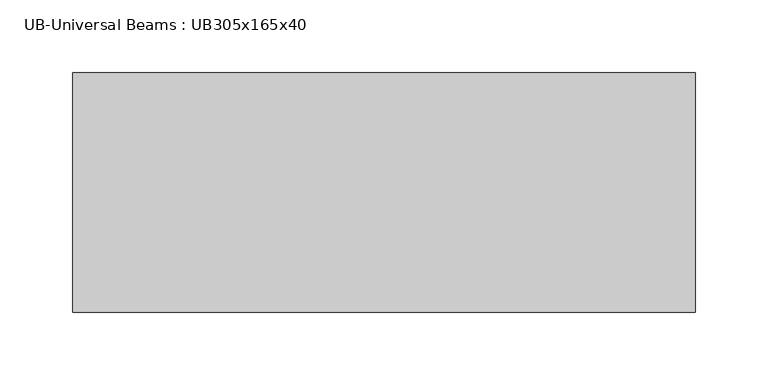
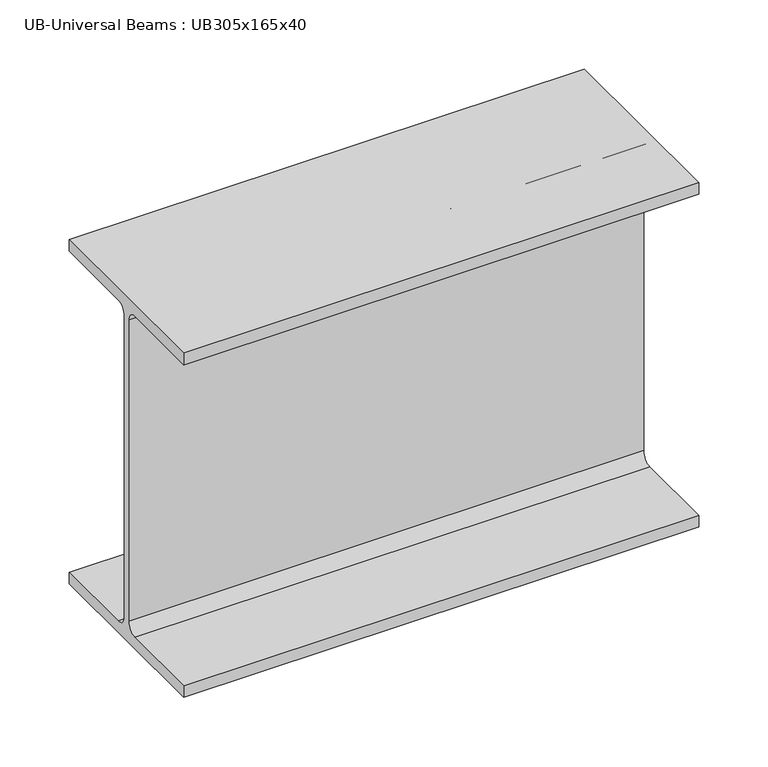
"""IFC4 building model written with IfcOpenShell, lengths in millimetres: beam geometry, UB-Universal Beams : UB305x165x40."""

from ifc_helpers import new_model, si_unit, point, frame, frame_2d, origin, place, context, project, spatial, polyline, circle_curve, trimmed, segment, composite_curve, outline, extrude, source, transform, mapped, element, save


def ub_universal_beams_ub305x165x40_c2ddfea9(model_context):
    return source(origin(), model_context, "Body", "SweptSolid", [
        extrude(outline(composite_curve([segment(polyline([(-82.5, -141.5), (-11.9, -141.5)]), True, "CONTINUOUS"), segment(trimmed(circle_curve(frame_2d((-11.9, -132.6)), 8.9), [point((-11.9, -141.5))], [point((-3.0, -132.6))], True, "CARTESIAN"), True, "CONTINUOUS"), segment(polyline([(-3.0, -132.6), (-3.0, 132.6)]), True, "CONTINUOUS"), segment(trimmed(circle_curve(frame_2d((-11.9, 132.6)), 8.9), [point((-3.0, 132.6))], [point((-11.9, 141.5))], True, "CARTESIAN"), True, "CONTINUOUS"), segment(polyline([(-11.9, 141.5), (-82.5, 141.5), (-82.5, 151.7), (82.5, 151.7), (82.5, 141.5), (11.9, 141.5)]), True, "CONTINUOUS"), segment(trimmed(circle_curve(frame_2d((11.9, 132.6)), 8.9), [point((11.9, 141.5))], [point((3.0, 132.6))], True, "CARTESIAN"), True, "CONTINUOUS"), segment(polyline([(3.0, 132.6), (3.0, -132.6)]), True, "CONTINUOUS"), segment(trimmed(circle_curve(frame_2d((11.9, -132.6)), 8.9), [point((3.0, -132.6))], [point((11.9, -141.5))], True, "CARTESIAN"), True, "CONTINUOUS"), segment(polyline([(11.9, -141.5), (82.5, -141.5), (82.5, -151.7), (-82.5, -151.7), (-82.5, -141.5)]), True, "CONTINUOUS")], self_intersect=False)), frame((368.4, 0.0, 0.0), z_axis=(1.0, 0.0, 0.0), x_axis=(0.0, 1.0, 0.0)), (0.0, 0.0, 1.0), 429.1),
    ])


if __name__ == "__main__":
    model = new_model("IFC4")
    model_context = context("Model", 3, world=origin())
    ifc_project = project(units=[si_unit("LENGTHUNIT", "METRE", prefix="MILLI")], contexts=[model_context])
    site = spatial("IfcSite", under=ifc_project)
    building = spatial("IfcBuilding", under=site)
    placement = place(None, origin())
    ub_universal_beams_ub305x165x40_shape = ub_universal_beams_ub305x165x40_c2ddfea9(model_context)
    element("IfcBeam", 1, ObjectType="UB-Universal Beams : UB305x165x40", at=placement, inside=building, context=model_context, shape_type="MappedRepresentation", body=[
        mapped(ub_universal_beams_ub305x165x40_shape, transform((0.0, 0.0, 0.0), x_axis=(1.0, 0.0, 0.0), y_axis=(0.0, 1.0, 0.0), z_axis=(0.0, 0.0, 1.0))),
    ])
    save(model, "model.ifc")

# Revit data of these elements
# Type "UB-Universal Beams : UB305x165x40"
#   Section Name Key = "UB305X165X40"
#   Width = 16.5 cm
#   Web Thickness = 0.6 cm
#   Web Fillet = 0.89 cm
#   Warping Constant = 164000.0 cm⁶
#   Torsional Moment of Inertia = 14.70 cm⁴
#   Section Area = 51.3 cm²
#   Plastic Modulus weak axis = 142.0 cm³
#   Plastic Modulus strong axis = 623.0 cm³
#   Nominal Weight = 40.2999 kgf/m
#   Moment of Inertia weak axis = 764.00 cm⁴
#   Moment of Inertia strong axis = 8503.00 cm⁴
#   Height = 30.34 cm
#   Flange Thickness = 1.02 cm
#   Elastic Modulus weak axis = 92.6 cm³
#   Elastic Modulus strong axis = 560.0 cm³
#   Centroid Vertical = 15.17 cm
#   Centroid Horizontal = 8.25 cm
#   Bolt Spacing = 9.0 cm
#   Length [instance default] = 1500 mm
#   Structural Material [instance default] = Metal - Steel 43-275
#   Type Comments = ""
#   Assembly Code = ""
# Element 1 (IfcBeam, "UB-Universal Beams : UB305x165x40")
#   Materials on its faces: "Metal - Steel 43-275"
# Materials
#   "Metal - Steel 43-275": class "Metal", colour RGB 247 247 247, transparency 0, Cost = 0
